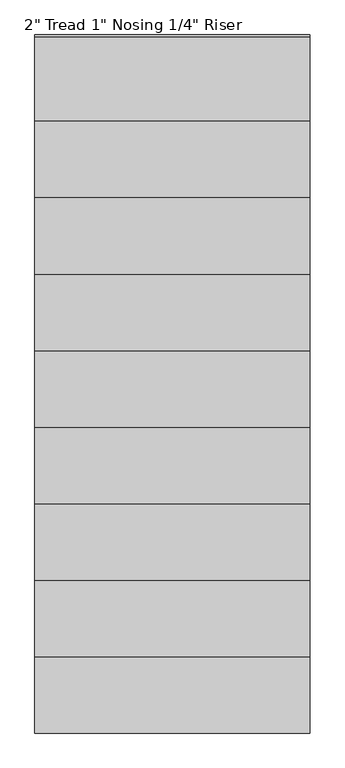
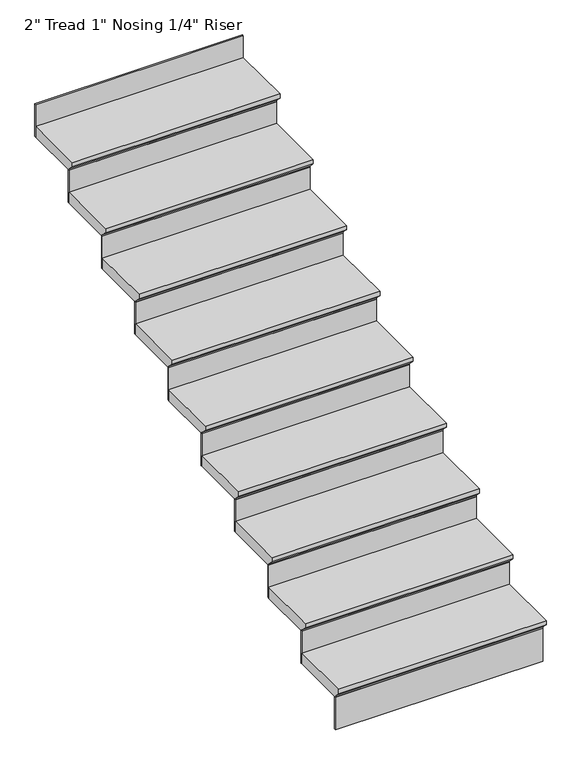
"""IFC4 building model written with IfcOpenShell, lengths in millimetres: stair flight geometry."""

from ifc_helpers import new_model, si_unit, frame, origin, place, context, project, spatial, polyline, outline, extrude, source, transform, mapped, element, save


def stair_flight_39a519ea(model_context):
    return source(origin(), model_context, "Body", "SweptSolid", [
        extrude(outline(polyline([(-6527.0593836, 1676.4), (-6247.6593836, 1676.4), (-6247.6593836, 1625.6), (-6501.6593836, 1625.6), (-6501.6593836, 1631.95), (-6527.0593836, 1657.35), (-6527.0593836, 1676.4)])), frame((-5280.3137331, 0.0, 0.0), z_axis=(1.0, 0.0, 0.0), x_axis=(0.0, 1.0, 0.0)), (0.0, 0.0, 1.0), 914.4),
        extrude(outline(polyline([(-4365.9137331, -6495.3093836), (-4365.9137331, -6501.6593836), (-5280.3137331, -6501.6593836), (-5280.3137331, -6495.3093836), (-4365.9137331, -6495.3093836)])), frame((0.0, 0.0, 1473.2), z_axis=(0.0, 0.0, 1.0), x_axis=(1.0, 0.0, 0.0)), (0.0, 0.0, 1.0), 152.4),
        extrude(outline(polyline([(-4365.9137331, -6241.3093836), (-4365.9137331, -6247.6593836), (-5280.3137331, -6247.6593836), (-5280.3137331, -6241.3093836), (-4365.9137331, -6241.3093836)])), frame((0.0, 0.0, 1625.6), z_axis=(0.0, 0.0, 1.0), x_axis=(1.0, 0.0, 0.0)), (0.0, 0.0, 1.0), 152.4),
        extrude(outline(polyline([(-6273.0593836, 1828.8), (-5993.6593836, 1828.8), (-5993.6593836, 1778.0), (-6247.6593836, 1778.0), (-6247.6593836, 1784.35), (-6273.0593836, 1809.75), (-6273.0593836, 1828.8)])), frame((-5280.3137331, 0.0, 0.0), z_axis=(1.0, 0.0, 0.0), x_axis=(0.0, 1.0, 0.0)), (0.0, 0.0, 1.0), 914.4),
        extrude(outline(polyline([(-4365.9137331, -5987.3093836), (-4365.9137331, -5993.6593836), (-5280.3137331, -5993.6593836), (-5280.3137331, -5987.3093836), (-4365.9137331, -5987.3093836)])), frame((0.0, 0.0, 1778.0), z_axis=(0.0, 0.0, 1.0), x_axis=(1.0, 0.0, 0.0)), (0.0, 0.0, 1.0), 152.4),
        extrude(outline(polyline([(-6019.0593836, 1981.2), (-5739.6593836, 1981.2), (-5739.6593836, 1930.4), (-5993.6593836, 1930.4), (-5993.6593836, 1936.75), (-6019.0593836, 1962.15), (-6019.0593836, 1981.2)])), frame((-5280.3137331, 0.0, 0.0), z_axis=(1.0, 0.0, 0.0), x_axis=(0.0, 1.0, 0.0)), (0.0, 0.0, 1.0), 914.4),
        extrude(outline(polyline([(-4365.9137331, -5733.3093836), (-4365.9137331, -5739.6593836), (-5280.3137331, -5739.6593836), (-5280.3137331, -5733.3093836), (-4365.9137331, -5733.3093836)])), frame((0.0, 0.0, 1930.4), z_axis=(0.0, 0.0, 1.0), x_axis=(1.0, 0.0, 0.0)), (0.0, 0.0, 1.0), 152.4),
        extrude(outline(polyline([(-5765.0593836, 2133.6), (-5485.6593836, 2133.6), (-5485.6593836, 2082.8), (-5739.6593836, 2082.8), (-5739.6593836, 2089.15), (-5765.0593836, 2114.55), (-5765.0593836, 2133.6)])), frame((-5280.3137331, 0.0, 0.0), z_axis=(1.0, 0.0, 0.0), x_axis=(0.0, 1.0, 0.0)), (0.0, 0.0, 1.0), 914.4),
        extrude(outline(polyline([(-4365.9137331, -5479.3093836), (-4365.9137331, -5485.6593836), (-5280.3137331, -5485.6593836), (-5280.3137331, -5479.3093836), (-4365.9137331, -5479.3093836)])), frame((0.0, 0.0, 2082.8), z_axis=(0.0, 0.0, 1.0), x_axis=(1.0, 0.0, 0.0)), (0.0, 0.0, 1.0), 152.4),
        extrude(outline(polyline([(-5511.0593836, 2286.0), (-5231.6593836, 2286.0), (-5231.6593836, 2235.2), (-5485.6593836, 2235.2), (-5485.6593836, 2241.55), (-5511.0593836, 2266.95), (-5511.0593836, 2286.0)])), frame((-5280.3137331, 0.0, 0.0), z_axis=(1.0, 0.0, 0.0), x_axis=(0.0, 1.0, 0.0)), (0.0, 0.0, 1.0), 914.4),
        extrude(outline(polyline([(-4365.9137331, -5225.3093836), (-4365.9137331, -5231.6593836), (-5280.3137331, -5231.6593836), (-5280.3137331, -5225.3093836), (-4365.9137331, -5225.3093836)])), frame((0.0, 0.0, 2235.2), z_axis=(0.0, 0.0, 1.0), x_axis=(1.0, 0.0, 0.0)), (0.0, 0.0, 1.0), 152.4),
        extrude(outline(polyline([(-5257.0593836, 2438.4), (-4977.6593836, 2438.4), (-4977.6593836, 2387.6), (-5231.6593836, 2387.6), (-5231.6593836, 2393.95), (-5257.0593836, 2419.35), (-5257.0593836, 2438.4)])), frame((-5280.3137331, 0.0, 0.0), z_axis=(1.0, 0.0, 0.0), x_axis=(0.0, 1.0, 0.0)), (0.0, 0.0, 1.0), 914.4),
        extrude(outline(polyline([(-4365.9137331, -4971.3093836), (-4365.9137331, -4977.6593836), (-5280.3137331, -4977.6593836), (-5280.3137331, -4971.3093836), (-4365.9137331, -4971.3093836)])), frame((0.0, 0.0, 2387.6), z_axis=(0.0, 0.0, 1.0), x_axis=(1.0, 0.0, 0.0)), (0.0, 0.0, 1.0), 152.4),
        extrude(outline(polyline([(-5003.0593836, 2590.8), (-4723.6593836, 2590.8), (-4723.6593836, 2540.0), (-4977.6593836, 2540.0), (-4977.6593836, 2546.35), (-5003.0593836, 2571.75), (-5003.0593836, 2590.8)])), frame((-5280.3137331, 0.0, 0.0), z_axis=(1.0, 0.0, 0.0), x_axis=(0.0, 1.0, 0.0)), (0.0, 0.0, 1.0), 914.4),
        extrude(outline(polyline([(-4365.9137331, -4717.3093836), (-4365.9137331, -4723.6593836), (-5280.3137331, -4723.6593836), (-5280.3137331, -4717.3093836), (-4365.9137331, -4717.3093836)])), frame((0.0, 0.0, 2540.0), z_axis=(0.0, 0.0, 1.0), x_axis=(1.0, 0.0, 0.0)), (0.0, 0.0, 1.0), 152.4),
        extrude(outline(polyline([(-4749.0593836, 2743.2), (-4469.6593836, 2743.2), (-4469.6593836, 2692.4), (-4723.6593836, 2692.4), (-4723.6593836, 2698.75), (-4749.0593836, 2724.15), (-4749.0593836, 2743.2)])), frame((-5280.3137331, 0.0, 0.0), z_axis=(1.0, 0.0, 0.0), x_axis=(0.0, 1.0, 0.0)), (0.0, 0.0, 1.0), 914.4),
        extrude(outline(polyline([(-4365.9137331, -4463.3093836), (-4365.9137331, -4469.6593836), (-5280.3137331, -4469.6593836), (-5280.3137331, -4463.3093836), (-4365.9137331, -4463.3093836)])), frame((0.0, 0.0, 2692.4), z_axis=(0.0, 0.0, 1.0), x_axis=(1.0, 0.0, 0.0)), (0.0, 0.0, 1.0), 152.4),
        extrude(outline(polyline([(-4365.9137331, -4209.3093836), (-4365.9137331, -4215.6593836), (-5280.3137331, -4215.6593836), (-5280.3137331, -4209.3093836), (-4365.9137331, -4209.3093836)])), frame((0.0, 0.0, 2844.8), z_axis=(0.0, 0.0, 1.0), x_axis=(1.0, 0.0, 0.0)), (0.0, 0.0, 1.0), 152.4),
        extrude(outline(polyline([(-4495.0593836, 2895.6), (-4215.6593836, 2895.6), (-4215.6593836, 2844.8), (-4469.6593836, 2844.8), (-4469.6593836, 2851.15), (-4495.0593836, 2876.55), (-4495.0593836, 2895.6)])), frame((-5280.3137331, 0.0, 0.0), z_axis=(1.0, 0.0, 0.0), x_axis=(0.0, 1.0, 0.0)), (0.0, 0.0, 1.0), 914.4),
    ])


if __name__ == "__main__":
    model = new_model("IFC4")
    model_context = context("Model", 3, world=origin())
    ifc_project = project(units=[si_unit("LENGTHUNIT", "METRE", prefix="MILLI")], contexts=[model_context])
    site = spatial("IfcSite", under=ifc_project)
    building = spatial("IfcBuilding", under=site)
    placement = place(None, origin())
    stair_flight_shape = stair_flight_39a519ea(model_context)
    element("IfcStairFlight", 1, ObjectType="2\" Tread 1\" Nosing 1/4\" Riser", at=placement, inside=building, context=model_context, shape_type="MappedRepresentation", body=[
        mapped(stair_flight_shape, transform((0.0, 0.0, 0.0), x_axis=(1.0, 0.0, 0.0), y_axis=(0.0, 1.0, 0.0), z_axis=(0.0, 0.0, 1.0))),
    ])
    save(model, "model.ifc")
